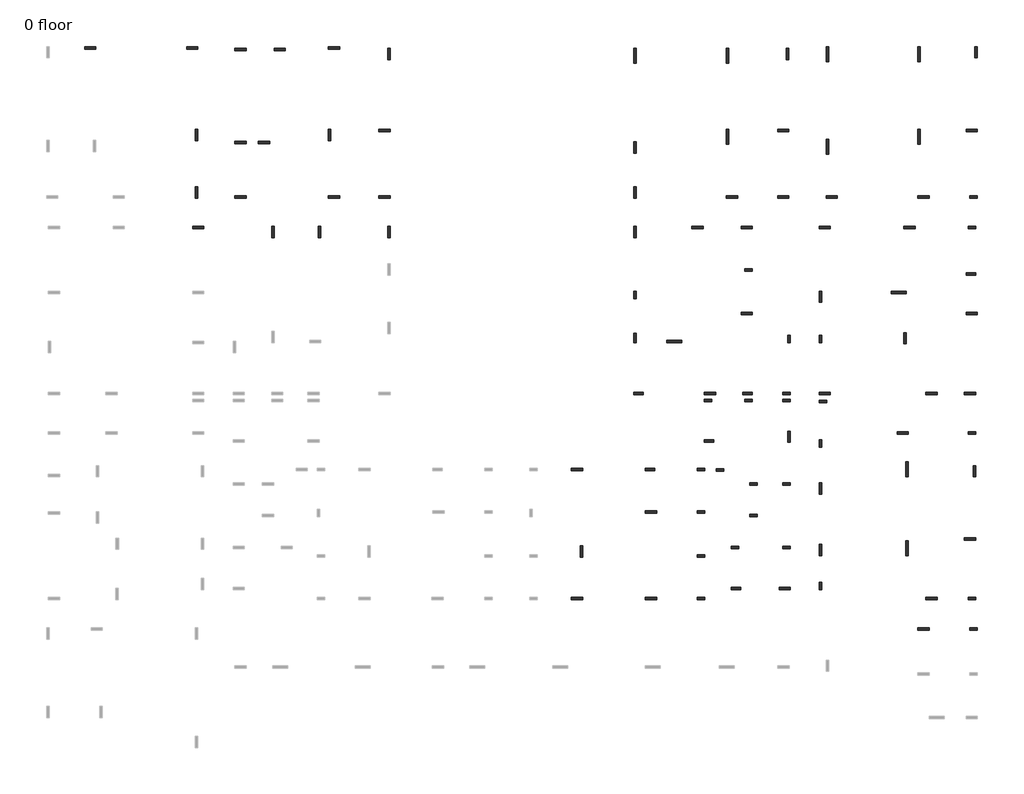
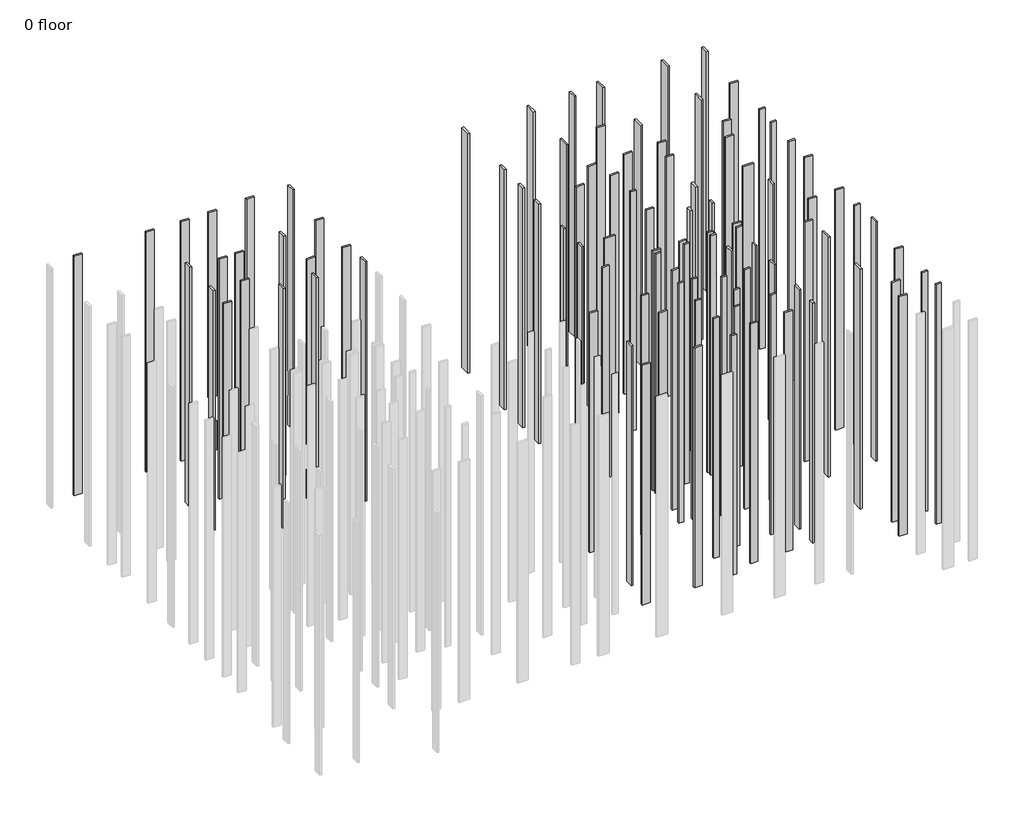
# One storey, part 2 of 2: 100 columns.
"""IFC4 building model written with IfcOpenShell, lengths in millimetres."""

from ifc_helpers import new_model, si_unit, frame, origin, origin_with_axes, place, context, project, spatial, polyline, outline, extrude, faceted_brep, transform, mapped, element, save
from components import column_6d4d5e46, column_25705251, column_7936e864, column_a28f250a

model = new_model("IFC4")

# Units and contexts
model_context = context("Model", 3, world=origin())
ifc_project = project(units=[si_unit("LENGTHUNIT", "METRE", prefix="MILLI")], contexts=[model_context])

# Site, building, storey
site = spatial("IfcSite", under=ifc_project)
building = spatial("IfcBuilding", under=site)
storey = spatial("IfcBuildingStorey", under=building, Name="0 floor", Elevation=0.0)

# Columns
placement = place(None, origin())
column_shape = column_6d4d5e46(model_context)
element("IfcColumn", 1, ObjectType="Rectangular Column : 2' x 8\"", at=placement, inside=storey, context=model_context, shape_type="MappedRepresentation", body=[
    mapped(column_shape, transform((32806.420549, 1766.0930615, 0.0), x_axis=(1.0, 0.0, 0.0), y_axis=(0.0, 1.0, 0.0), z_axis=(0.0, 0.0, 1.0))),
])
element("IfcColumn", 2, ObjectType="Rectangular Column : 2' x 8\"", at=placement, inside=storey, context=model_context, shape_type="MappedRepresentation", body=[
    mapped(column_shape, transform((10708.4180594, 14707.393062, 0.0), x_axis=(1.0, 0.0, 0.0), y_axis=(0.0, 1.0, 0.0), z_axis=(0.0, 0.0, 1.0))),
])
element("IfcColumn", 3, ObjectType="Rectangular Column : 2' x 8\"", at=placement, inside=storey, context=model_context, shape_type="MappedRepresentation", body=[
    mapped(column_shape, transform((10708.420549, 11265.693062, 0.0), x_axis=(-1.0, 0.0, 0.0), y_axis=(0.0, -1.0, 0.0), z_axis=(0.0, 0.0, 1.0))),
])
element("IfcColumn", 4, ObjectType="Rectangular Column : 2' x 8\"", at=placement, inside=storey, context=model_context, shape_type="MappedRepresentation", body=[
    mapped(column_shape, transform((10708.420549, 4255.2930586, 0.0), x_axis=(-1.0, 0.0, 0.0), y_axis=(0.0, -1.0, 0.0), z_axis=(0.0, 0.0, 1.0))),
])
element("IfcColumn", 5, ObjectType="Rectangular Column : 2' x 8\"", at=placement, inside=storey, context=model_context, shape_type="MappedRepresentation", body=[
    mapped(column_shape, transform((10708.420549, 7709.5953697, 0.0), x_axis=(-1.0, 0.0, 0.0), y_axis=(0.0, -1.0, 0.0), z_axis=(0.0, 0.0, 1.0))),
])
element("IfcColumn", 6, ObjectType="Rectangular Column : 2' x 8\"", at=placement, inside=storey, context=model_context, shape_type="MappedRepresentation", body=[
    mapped(column_shape, transform((13454.4520067, 8408.1930618, 0.0), x_axis=(1.0, 0.0, 0.0), y_axis=(0.0, 1.0, 0.0), z_axis=(0.0, 0.0, 1.0))),
])
element("IfcColumn", 7, ObjectType="Rectangular Column : 2' x 8\"", at=placement, inside=storey, context=model_context, shape_type="MappedRepresentation", body=[
    mapped(column_shape, transform((17645.4520067, 8408.1930618, 0.0), x_axis=(1.0, 0.0, 0.0), y_axis=(0.0, 1.0, 0.0), z_axis=(0.0, 0.0, 1.0))),
])
element("IfcColumn", 8, ObjectType="Rectangular Column : 2' x 8\"", at=placement, inside=storey, context=model_context, shape_type="MappedRepresentation", body=[
    mapped(column_shape, transform((14962.920549, 13538.9930617, 0.0), x_axis=(1.0, 0.0, 0.0), y_axis=(0.0, 1.0, 0.0), z_axis=(0.0, 0.0, 1.0))),
])
element("IfcColumn", 9, ObjectType="Rectangular Column : 2' x 8\"", at=placement, inside=storey, context=model_context, shape_type="MappedRepresentation", body=[
    mapped(column_shape, transform((14962.920549, 10986.2930571, 0.0), x_axis=(1.0, 0.0, 0.0), y_axis=(0.0, 1.0, 0.0), z_axis=(0.0, 0.0, 1.0))),
])
element("IfcColumn", 10, ObjectType="Rectangular Column : 2' x 8\"", at=placement, inside=storey, context=model_context, shape_type="MappedRepresentation", body=[
    mapped(column_shape, transform((17645.4520067, 13538.9930617, 0.0), x_axis=(1.0, 0.0, 0.0), y_axis=(0.0, 1.0, 0.0), z_axis=(0.0, 0.0, 1.0))),
])
element("IfcColumn", 11, ObjectType="Rectangular Column : 2' x 8\"", at=placement, inside=storey, context=model_context, shape_type="MappedRepresentation", body=[
    mapped(column_shape, transform((12235.2520067, 14681.993062, 0.0), x_axis=(1.0, 0.0, 0.0), y_axis=(0.0, 1.0, 0.0), z_axis=(0.0, 0.0, 1.0))),
])
element("IfcColumn", 12, ObjectType="Rectangular Column : 2' x 8\"", at=placement, inside=storey, context=model_context, shape_type="MappedRepresentation", body=[
    mapped(column_shape, transform((11282.7520067, 20308.093062, 0.0), x_axis=(1.0, 0.0, 0.0), y_axis=(0.0, 1.0, 0.0), z_axis=(0.0, 0.0, 1.0))),
])
element("IfcColumn", 13, ObjectType="Rectangular Column : 2' x 8\"", at=placement, inside=storey, context=model_context, shape_type="MappedRepresentation", body=[
    mapped(column_shape, transform((14556.520549, 20308.093062, 0.0), x_axis=(1.0, 0.0, 0.0), y_axis=(0.0, 1.0, 0.0), z_axis=(0.0, 0.0, 1.0))),
])
element("IfcColumn", 14, ObjectType="Rectangular Column : 2' x 8\"", at=placement, inside=storey, context=model_context, shape_type="MappedRepresentation", body=[
    mapped(column_shape, transform((17642.6205489, 20892.2930623, 0.0), x_axis=(1.0, 0.0, 0.0), y_axis=(0.0, 1.0, 0.0), z_axis=(0.0, 0.0, 1.0))),
])
element("IfcColumn", 15, ObjectType="Rectangular Column : 2' x 8\"", at=placement, inside=storey, context=model_context, shape_type="MappedRepresentation", body=[
    mapped(column_shape, transform((17642.618059, 20308.093062, 0.0), x_axis=(1.0, 0.0, 0.0), y_axis=(0.0, 1.0, 0.0), z_axis=(0.0, 0.0, 1.0))),
])
element("IfcColumn", 16, ObjectType="Rectangular Column : 2' x 8\"", at=placement, inside=storey, context=model_context, shape_type="MappedRepresentation", body=[
    mapped(column_shape, transform((5361.720549, 28867.8930624, 0.0), x_axis=(0.0, 1.0, 0.0), y_axis=(-1.0, 0.0, 0.0), z_axis=(0.0, 0.0, 1.0))),
])
element("IfcColumn", 17, ObjectType="Rectangular Column : 2' x 8\"", at=placement, inside=storey, context=model_context, shape_type="MappedRepresentation", body=[
    mapped(column_shape, transform((14556.520549, 30899.893062, 0.0), x_axis=(1.0, 0.0, 0.0), y_axis=(0.0, 1.0, 0.0), z_axis=(0.0, 0.0, 1.0))),
])
element("IfcColumn", 18, ObjectType="Rectangular Column : 2' x 8\"", at=placement, inside=storey, context=model_context, shape_type="MappedRepresentation", body=[
    mapped(column_shape, transform((17845.820549, 25311.8930465, 0.0), x_axis=(0.0, 1.0, 0.0), y_axis=(-1.0, 0.0, 0.0), z_axis=(0.0, 0.0, 1.0))),
])
element("IfcColumn", 19, ObjectType="Rectangular Column : 2' x 8\"", at=placement, inside=storey, context=model_context, shape_type="MappedRepresentation", body=[
    mapped(column_shape, transform((32654.0205491, 4255.2930626, 0.0), x_axis=(1.0, 0.0, 0.0), y_axis=(0.0, 1.0, 0.0), z_axis=(0.0, 0.0, 1.0))),
])
element("IfcColumn", 20, ObjectType="Rectangular Column : 2' x 8\"", at=placement, inside=storey, context=model_context, shape_type="MappedRepresentation", body=[
    mapped(column_shape, transform((32654.020549, 17679.1930626, 0.0), x_axis=(1.0, 0.0, 0.0), y_axis=(0.0, 1.0, 0.0), z_axis=(0.0, 0.0, 1.0))),
])
element("IfcColumn", 21, ObjectType="Rectangular Column : 2' x 8\"", at=placement, inside=storey, context=model_context, shape_type="MappedRepresentation", body=[
    mapped(column_shape, transform((32654.0205491, 34316.1930593, 0.0), x_axis=(1.0, 0.0, 0.0), y_axis=(0.0, 1.0, 0.0), z_axis=(0.0, 0.0, 1.0))),
])
element("IfcColumn", 22, ObjectType="Rectangular Column : 2' x 8\"", at=placement, inside=storey, context=model_context, shape_type="MappedRepresentation", body=[
    mapped(column_shape, transform((20586.1915809, 20244.5930606, 0.0), x_axis=(1.0, 0.0, 0.0), y_axis=(0.0, 1.0, 0.0), z_axis=(0.0, 0.0, 1.0))),
])
element("IfcColumn", 23, ObjectType="Rectangular Column : 2' x 8\"", at=placement, inside=storey, context=model_context, shape_type="MappedRepresentation", body=[
    mapped(column_shape, transform((20373.120549, 16802.893062, 0.0), x_axis=(0.0, 1.0, 0.0), y_axis=(-1.0, 0.0, 0.0), z_axis=(0.0, 0.0, 1.0))),
])
element("IfcColumn", 24, ObjectType="Rectangular Column : 2' x 8\"", at=placement, inside=storey, context=model_context, shape_type="MappedRepresentation", body=[
    mapped(column_shape, transform((20373.120549, 5283.9930634, 0.0), x_axis=(0.0, 1.0, 0.0), y_axis=(-1.0, 0.0, 0.0), z_axis=(0.0, 0.0, 1.0))),
])
element("IfcColumn", 25, ObjectType="Rectangular Column : 2' x 8\"", at=placement, inside=storey, context=model_context, shape_type="MappedRepresentation", body=[
    mapped(column_shape, transform((20373.120549, 25311.8930566, 0.0), x_axis=(0.0, 1.0, 0.0), y_axis=(-1.0, 0.0, 0.0), z_axis=(0.0, 0.0, 1.0))),
])
element("IfcColumn", 26, ObjectType="Rectangular Column : 2' x 8\"", at=placement, inside=storey, context=model_context, shape_type="MappedRepresentation", body=[
    mapped(column_shape, transform((32806.420549, 36805.393062, 0.0), x_axis=(1.0, 0.0, 0.0), y_axis=(0.0, 1.0, 0.0), z_axis=(0.0, 0.0, 1.0))),
])
column_2_shape = column_25705251(model_context)
element("IfcColumn", 27, ObjectType="Rectangular Column : 8\" x 2'6\"", at=placement, inside=storey, context=model_context, shape_type="MappedRepresentation", body=[
    mapped(column_2_shape, transform((6568.220549, 14706.9955039, 0.0), x_axis=(1.0, 0.0, 0.0), y_axis=(0.0, 1.0, 0.0), z_axis=(0.0, 0.0, 1.0))),
])
element("IfcColumn", 28, ObjectType="Rectangular Column : 8\" x 2'6\"", at=placement, inside=storey, context=model_context, shape_type="MappedRepresentation", body=[
    mapped(column_2_shape, transform((13530.6520067, 5080.7930619, 0.0), x_axis=(1.0, 0.0, 0.0), y_axis=(0.0, 1.0, 0.0), z_axis=(0.0, 0.0, 1.0))),
])
element("IfcColumn", 29, ObjectType="Rectangular Column : 8\" x 2'6\"", at=placement, inside=storey, context=model_context, shape_type="MappedRepresentation", body=[
    mapped(column_2_shape, transform((11358.9520067, 17006.093062, 0.0), x_axis=(1.0, 0.0, 0.0), y_axis=(0.0, 1.0, 0.0), z_axis=(0.0, 0.0, 1.0))),
])
element("IfcColumn", 30, ObjectType="Rectangular Column : 8\" x 2'6\"", at=placement, inside=storey, context=model_context, shape_type="MappedRepresentation", body=[
    mapped(column_2_shape, transform((14480.3205488, 20892.2930623, 0.0), x_axis=(1.0, 0.0, 0.0), y_axis=(0.0, 1.0, 0.0), z_axis=(0.0, 0.0, 1.0))),
])
element("IfcColumn", 31, ObjectType="Rectangular Column : 8\" x 2'6\"", at=placement, inside=storey, context=model_context, shape_type="MappedRepresentation", body=[
    mapped(column_2_shape, transform((5361.720549, 25388.093059, 0.0), x_axis=(0.0, 1.0, 0.0), y_axis=(-1.0, 0.0, 0.0), z_axis=(0.0, 0.0, 1.0))),
])
element("IfcColumn", 32, ObjectType="Rectangular Column : 8\" x 2'6\"", at=placement, inside=storey, context=model_context, shape_type="MappedRepresentation", body=[
    mapped(column_2_shape, transform((5641.120549, 20892.2930623, 0.0), x_axis=(-1.0, 0.0, 0.0), y_axis=(0.0, -1.0, 0.0), z_axis=(0.0, 0.0, 1.0))),
])
element("IfcColumn", 33, ObjectType="Rectangular Column : 8\" x 2'6\"", at=placement, inside=storey, context=model_context, shape_type="MappedRepresentation", body=[
    mapped(column_2_shape, transform((32577.8205488, 30569.6930587, 0.0), x_axis=(1.0, 0.0, 0.0), y_axis=(0.0, 1.0, 0.0), z_axis=(0.0, 0.0, 1.0))),
])
element("IfcColumn", 34, ObjectType="Rectangular Column : 8\" x 3'", at=placement, inside=storey, context=model_context, shape_type="SweptSolid", body=[
    extrude(outline(polyline([(-23004.2428642, 48850.8496871), (-23004.2428642, 48647.6496871), (-23918.6428642, 48647.6496871), (-23918.6428642, 48850.8496871), (-23004.2428642, 48850.8496871)])), origin_with_axes(), (0.0, 0.0, 1.0), 3505.2),
    extrude(outline(polyline([(-23004.2428642, 48850.8496871), (-23004.2428642, 48647.6496871), (-23918.6428642, 48647.6496871), (-23918.6428642, 48850.8496871), (-23004.2428642, 48850.8496871)])), frame((0.0, 0.0, 6553.2), z_axis=(0.0, 0.0, 1.0), x_axis=(1.0, 0.0, 0.0)), (0.0, 0.0, 1.0), 22555.2),
])
element("IfcColumn", 35, ObjectType="Rectangular Column : 8\" x 3'", at=placement, inside=storey, context=model_context, shape_type="Brep", body=[
    faceted_brep([(-26166.5159189, 48850.883515, 0.0), (-26166.5159189, 48647.683515, 0.0), (-27080.9159189, 48647.683515, 0.0), (-27080.9159189, 48850.883515, 0.0), (-26166.5159189, 48850.883515, 29108.4), (-26166.5159189, 48647.683515, 29108.4), (-26166.5159189, 48647.683515, 6553.2), (-26166.5159189, 48647.683515, 3505.2), (-26166.5159189, 48850.883515, 3505.2), (-26166.5159189, 48850.883515, 6553.2), (-27080.9159189, 48647.683515, 29108.4), (-27080.9159189, 48850.883515, 29108.4)], [[[0, 1, 2, 3]], [[4, 5, 6, 7, 1, 0, 8, 9]], [[5, 10, 2, 1, 7, 6]], [[10, 11, 3, 2]], [[11, 4, 9, 8, 0, 3]], [[4, 11, 10, 5]]]),
])
element("IfcColumn", 36, ObjectType="Rectangular Column : 8\" x 3'", at=placement, inside=storey, context=model_context, shape_type="Brep", body=[
    faceted_brep([(-18587.4473751, 49003.2834458, 0.0), (-18587.4473751, 48800.0834458, 0.0), (-19501.8473751, 48800.0834458, 0.0), (-19501.8473751, 49003.2834458, 0.0), (-18587.4473751, 49003.2834458, 29108.4), (-18587.4473751, 48800.0834458, 29108.4), (-19501.8473751, 48800.0834458, 29108.4), (-19501.8473751, 49003.2834458, 29108.4), (-19501.8473751, 49003.2834458, 6553.2), (-19501.8473751, 49003.2834458, 3505.2)], [[[0, 1, 2, 3]], [[4, 5, 1, 0]], [[5, 6, 2, 1]], [[6, 7, 8, 9, 3, 2]], [[7, 4, 0, 3, 9, 8]], [[4, 7, 6, 5]]]),
])
element("IfcColumn", 37, ObjectType="Rectangular Column : 8\" x 3'", at=placement, inside=storey, context=model_context, shape_type="Brep", body=[
    faceted_brep([(-14713.9473752, 48850.8834491, 0.0), (-14510.7473752, 48850.8834491, 0.0), (-14510.7473752, 47936.4834491, 0.0), (-14713.9473752, 47936.4834491, 0.0), (-14713.9473752, 48850.8834491, 29108.4), (-14510.7473752, 48850.8834491, 29108.4), (-14510.7473752, 48850.8834491, 6553.2), (-14713.9473752, 48850.8834491, 6553.2), (-14510.7473752, 48850.8834491, 3505.2), (-14510.7473752, 48749.2834491, 3505.2), (-14510.7473752, 48749.2834491, 6553.2), (-14510.7473752, 47936.4834491, 29108.4), (-14510.7473752, 47936.4834491, 6553.2), (-14510.7473752, 47936.4834491, 3505.2), (-14713.9473752, 47936.4834491, 29108.4), (-14713.9473752, 47936.4834491, 6553.2), (-14713.9473752, 47936.4834491, 3505.2), (-14713.9473752, 48749.2834491, 6553.2), (-14713.9473752, 48749.2834491, 3505.2), (-14713.9473752, 48850.8834491, 3505.2)], [[[0, 1, 2, 3]], [[4, 5, 6, 7]], [[2, 1, 8, 9, 10, 6, 5, 11, 12, 13]], [[3, 2, 13, 12, 11, 14, 15, 16]], [[0, 3, 16, 15, 14, 4, 7, 17, 18, 19]], [[5, 4, 14, 11]], [[18, 9, 8, 19]], [[10, 17, 7, 6]], [[9, 18, 17, 10]], [[1, 0, 19, 8]]]),
])
element("IfcColumn", 38, ObjectType="Rectangular Column : 8\" x 3'", at=placement, inside=storey, context=model_context, shape_type="Brep", body=[
    faceted_brep([(-19501.8473752, 42291.7930622, 0.0), (-19298.6473752, 42291.7930622, 0.0), (-19298.6473752, 41377.3930622, 0.0), (-19501.8473752, 41377.3930622, 0.0), (-19501.8473752, 42291.7930622, 29108.4), (-19298.6473752, 42291.7930622, 29108.4), (-19298.6473752, 41377.3930622, 29108.4), (-19501.8473752, 41377.3930622, 29108.4), (-19501.8473752, 41377.3930622, 6553.2), (-19501.8473752, 41377.3930622, 3505.2)], [[[0, 1, 2, 3]], [[4, 5, 1, 0]], [[5, 6, 2, 1]], [[6, 7, 8, 9, 3, 2]], [[7, 4, 0, 3, 9, 8]], [[4, 7, 6, 5]]]),
])
element("IfcColumn", 39, ObjectType="Rectangular Column : 8\" x 3'", at=placement, inside=storey, context=model_context, shape_type="Brep", body=[
    faceted_brep([(-27080.9159175, 41110.6930626, 0.0), (-27080.9159175, 41313.8930626, 0.0), (-26166.5159175, 41313.8930626, 0.0), (-26166.5159175, 41110.6930626, 0.0), (-27080.9159175, 41110.6930626, 29108.4), (-27080.9159175, 41313.8930626, 29108.4), (-27080.9159175, 41313.8930626, 6553.2), (-27080.9159175, 41313.8930626, 3505.2), (-27080.9159175, 41110.6930626, 3505.2), (-27080.9159175, 41110.6930626, 6553.2), (-26166.5159175, 41313.8930626, 29108.4), (-26166.5159175, 41110.6930626, 29108.4)], [[[0, 1, 2, 3]], [[4, 5, 6, 7, 1, 0, 8, 9]], [[5, 10, 2, 1, 7, 6]], [[10, 11, 3, 2]], [[11, 4, 9, 8, 0, 3]], [[4, 11, 10, 5]]]),
])
element("IfcColumn", 40, ObjectType="Rectangular Column : 8\" x 3'", at=placement, inside=storey, context=model_context, shape_type="Brep", body=[
    faceted_brep([(-25175.9159175, 41110.693059, 0.0), (-25175.9159175, 41313.893059, 0.0), (-24261.5159175, 41313.893059, 0.0), (-24261.5159175, 41110.693059, 0.0), (-25175.9159175, 41110.693059, 29108.4), (-25175.9159175, 41313.893059, 29108.4), (-25175.9159175, 41110.693059, 3505.2), (-25175.9159175, 41110.693059, 6553.2), (-24261.5159175, 41313.893059, 29108.4), (-24261.5159175, 41110.693059, 29108.4), (-24261.5159175, 41110.693059, 6553.2), (-24261.5159175, 41110.693059, 3505.2)], [[[0, 1, 2, 3]], [[4, 5, 1, 0, 6, 7]], [[5, 8, 2, 1]], [[8, 9, 10, 11, 3, 2]], [[9, 4, 7, 6, 0, 3, 11, 10]], [[4, 9, 8, 5]]]),
])
element("IfcColumn", 41, ObjectType="Rectangular Column : 8\" x 3'", at=placement, inside=storey, context=model_context, shape_type="Brep", body=[
    faceted_brep([(-15425.1473762, 42088.593059, 0.0), (-15425.1473762, 42291.793059, 0.0), (-14510.7473762, 42291.793059, 0.0), (-14510.7473762, 42088.593059, 0.0), (-15425.1473762, 42088.593059, 29108.4), (-15425.1473762, 42291.793059, 29108.4), (-15425.1473762, 42291.793059, 6553.2), (-15425.1473762, 42291.793059, 3505.2), (-14510.7473762, 42291.793059, 29108.4), (-14510.7473762, 42291.793059, 6553.2), (-14713.9473752, 42291.793059, 6553.2), (-14713.9473752, 42291.793059, 3505.2), (-14510.7473762, 42291.793059, 3505.2), (-14510.7473762, 42190.193059, 3505.2), (-14510.7473762, 42190.193059, 6553.2), (-14510.7473762, 42088.593059, 29108.4), (-14510.7473762, 42088.593059, 6553.2), (-14510.7473762, 42088.593059, 3505.2), (-14713.9473752, 42190.193059, 6553.2), (-14713.9473752, 42190.193059, 3505.2)], [[[0, 1, 2, 3]], [[1, 0, 4, 5, 6, 7]], [[2, 1, 7, 6, 5, 8, 9, 10, 11, 12]], [[3, 2, 12, 13, 14, 9, 8, 15, 16, 17]], [[0, 3, 17, 16, 15, 4]], [[5, 4, 15, 8]], [[18, 19, 11, 10]], [[19, 13, 12, 11]], [[14, 18, 10, 9]], [[19, 18, 14, 13]]]),
])
element("IfcColumn", 42, ObjectType="Rectangular Column : 8\" x 3'", at=placement, inside=storey, context=model_context, shape_type="Brep", body=[
    faceted_brep([(-15425.1473752, 36703.793059, 0.0), (-15425.1473752, 36906.993059, 0.0), (-14510.7473752, 36906.993059, 0.0), (-14510.7473752, 36703.793059, 0.0), (-15425.1473752, 36703.793059, 29108.4), (-15425.1473752, 36906.993059, 29108.4), (-15425.1473752, 36906.993059, 6553.2), (-15425.1473752, 36906.993059, 3505.2), (-15425.1473752, 36703.793059, 3505.2), (-15425.1473752, 36703.793059, 6553.2), (-14510.7473752, 36906.993059, 29108.4), (-14510.7473752, 36703.793059, 29108.4)], [[[0, 1, 2, 3]], [[4, 5, 6, 7, 1, 0, 8, 9]], [[5, 10, 2, 1, 7, 6]], [[10, 11, 3, 2]], [[11, 4, 9, 8, 0, 3]], [[4, 11, 10, 5]]]),
])
element("IfcColumn", 43, ObjectType="Rectangular Column : 8\" x 3'", at=placement, inside=storey, context=model_context, shape_type="Brep", body=[
    faceted_brep([(-19501.8473751, 36703.793059, 0.0), (-19501.8473751, 36906.993059, 0.0), (-18587.4473751, 36906.993059, 0.0), (-18587.4473751, 36703.793059, 0.0), (-19501.8473751, 36703.793059, 29108.4), (-19501.8473751, 36906.993059, 29108.4), (-19501.8473751, 36906.993059, 6553.2), (-19501.8473751, 36703.793059, 6553.2), (-19501.8473751, 36906.993059, 3505.2), (-19400.2473752, 36906.993059, 3505.2), (-19400.2473752, 36906.993059, 6553.2), (-18587.4473751, 36906.993059, 29108.4), (-18587.4473751, 36906.993059, 6553.2), (-18587.4473751, 36906.993059, 3505.2), (-18587.4473751, 36703.793059, 29108.4), (-18587.4473751, 36703.793059, 6553.2), (-18587.4473751, 36703.793059, 3505.2), (-19400.2473752, 36703.793059, 6553.2), (-19400.2473752, 36703.793059, 3505.2), (-19501.8473751, 36703.793059, 3505.2)], [[[0, 1, 2, 3]], [[4, 5, 6, 7]], [[2, 1, 8, 9, 10, 6, 5, 11, 12, 13]], [[3, 2, 13, 12, 11, 14, 15, 16]], [[0, 3, 16, 15, 14, 4, 7, 17, 18, 19]], [[5, 4, 14, 11]], [[18, 9, 8, 19]], [[10, 17, 7, 6]], [[9, 18, 17, 10]], [[1, 0, 19, 8]]]),
])
element("IfcColumn", 44, ObjectType="Rectangular Column : 8\" x 3'", at=placement, inside=storey, context=model_context, shape_type="Brep", body=[
    faceted_brep([(-27080.9159175, 36703.793059, 0.0), (-27080.9159175, 36906.993059, 0.0), (-26166.5159175, 36906.993059, 0.0), (-26166.5159175, 36703.793059, 0.0), (-27080.9159175, 36703.793059, 29108.4), (-27080.9159175, 36906.993059, 29108.4), (-27080.9159175, 36906.993059, 6553.2), (-27080.9159175, 36906.993059, 3505.2), (-26166.5159175, 36906.993059, 29108.4), (-26166.5159175, 36906.993059, 6553.2), (-26166.5159175, 36906.993059, 3505.2), (-26166.5159175, 36703.793059, 29108.4), (-26166.5159175, 36703.793059, 6553.2), (-26166.5159175, 36703.793059, 3505.2)], [[[0, 1, 2, 3]], [[4, 5, 6, 7, 1, 0]], [[5, 8, 9, 10, 2, 1, 7, 6]], [[8, 11, 12, 13, 3, 2, 10, 9]], [[11, 4, 0, 3, 13, 12]], [[4, 11, 8, 5]]]),
])
column_3_shape = column_7936e864(model_context)
element("IfcColumn", 45, ObjectType="Rectangular Column : 8\" x 3'", at=placement, inside=storey, context=model_context, shape_type="MappedRepresentation", body=[
    mapped(column_3_shape, transform((-30548.0159175, 48895.7926361, 0.0), x_axis=(1.0, 0.0, 0.0), y_axis=(0.0, 1.0, 0.0), z_axis=(0.0, 0.0, 1.0))),
])
element("IfcColumn", 46, ObjectType="Rectangular Column : 8\" x 3'", at=placement, inside=storey, context=model_context, shape_type="MappedRepresentation", body=[
    mapped(column_3_shape, transform((-38812.8844599, 48895.793059, 0.0), x_axis=(1.0, 0.0, 0.0), y_axis=(0.0, 1.0, 0.0), z_axis=(0.0, 0.0, 1.0))),
])
element("IfcColumn", 47, ObjectType="Rectangular Column : 8\" x 3'", at=placement, inside=storey, context=model_context, shape_type="MappedRepresentation", body=[
    mapped(column_3_shape, transform((-30192.4159175, 41834.5930622, 0.0), x_axis=(0.0, 1.0, 0.0), y_axis=(-1.0, 0.0, 0.0), z_axis=(0.0, 0.0, 1.0))),
])
element("IfcColumn", 48, ObjectType="Rectangular Column : 8\" x 3'", at=placement, inside=storey, context=model_context, shape_type="MappedRepresentation", body=[
    mapped(column_3_shape, transform((-30192.4159175, 37160.993059, 0.0), x_axis=(0.0, -1.0, 0.0), y_axis=(1.0, 0.0, 0.0), z_axis=(0.0, 0.0, 1.0))),
])
element("IfcColumn", 49, ObjectType="Rectangular Column : 8\" x 3'", at=placement, inside=storey, context=model_context, shape_type="MappedRepresentation", body=[
    mapped(column_3_shape, transform((-30058.579451, 34316.1930586, 0.0), x_axis=(1.0, 0.0, 0.0), y_axis=(0.0, 1.0, 0.0), z_axis=(0.0, 0.0, 1.0))),
])
element("IfcColumn", 50, ObjectType="Rectangular Column : 8\" x 3'", at=placement, inside=storey, context=model_context, shape_type="MappedRepresentation", body=[
    mapped(column_3_shape, transform((-24010.3473751, 33960.5930622, 0.0), x_axis=(0.0, -1.0, 0.0), y_axis=(1.0, 0.0, 0.0), z_axis=(0.0, 0.0, 1.0))),
])
element("IfcColumn", 51, ObjectType="Rectangular Column : 8\" x 3'", at=placement, inside=storey, context=model_context, shape_type="MappedRepresentation", body=[
    mapped(column_3_shape, transform((-20213.0473751, 33960.5930622, 0.0), x_axis=(0.0, -1.0, 0.0), y_axis=(1.0, 0.0, 0.0), z_axis=(0.0, 0.0, 1.0))),
])
element("IfcColumn", 52, ObjectType="Rectangular Column : 8\" x 3'", at=placement, inside=storey, context=model_context, shape_type="MappedRepresentation", body=[
    mapped(column_3_shape, transform((-14612.3473751, 33960.5930622, 0.0), x_axis=(0.0, -1.0, 0.0), y_axis=(1.0, 0.0, 0.0), z_axis=(0.0, 0.0, 1.0))),
])
element("IfcColumn", 53, ObjectType="Rectangular Column : 8\" x 3'", at=placement, inside=storey, context=model_context, shape_type="MappedRepresentation", body=[
    mapped(column_3_shape, transform((28729.720549, 1766.0930615, 0.0), x_axis=(1.0, 0.0, 0.0), y_axis=(0.0, 1.0, 0.0), z_axis=(0.0, 0.0, 1.0))),
])
element("IfcColumn", 54, ObjectType="Rectangular Column : 8\" x 3'", at=placement, inside=storey, context=model_context, shape_type="MappedRepresentation", body=[
    mapped(column_3_shape, transform((650.020549, 14707.393062, 0.0), x_axis=(-1.0, 0.0, 0.0), y_axis=(0.0, -1.0, 0.0), z_axis=(0.0, 0.0, 1.0))),
])
element("IfcColumn", 55, ObjectType="Rectangular Column : 8\" x 3'", at=placement, inside=storey, context=model_context, shape_type="MappedRepresentation", body=[
    mapped(column_3_shape, transform((1005.620549, 8065.2930636, 0.0), x_axis=(0.0, -1.0, 0.0), y_axis=(1.0, 0.0, 0.0), z_axis=(0.0, 0.0, 1.0))),
])
element("IfcColumn", 56, ObjectType="Rectangular Column : 8\" x 3'", at=placement, inside=storey, context=model_context, shape_type="MappedRepresentation", body=[
    mapped(column_3_shape, transform((650.0205489, 4255.293062, 0.0), x_axis=(1.0, 0.0, 0.0), y_axis=(0.0, 1.0, 0.0), z_axis=(0.0, 0.0, 1.0))),
])
element("IfcColumn", 57, ObjectType="Rectangular Column : 8\" x 3'", at=placement, inside=storey, context=model_context, shape_type="MappedRepresentation", body=[
    mapped(column_3_shape, transform((6644.4205495, 4255.2930614, 0.0), x_axis=(1.0, 0.0, 0.0), y_axis=(0.0, 1.0, 0.0), z_axis=(0.0, 0.0, 1.0))),
])
element("IfcColumn", 58, ObjectType="Rectangular Column : 8\" x 3'", at=placement, inside=storey, context=model_context, shape_type="MappedRepresentation", body=[
    mapped(column_3_shape, transform((6647.2520062, 11265.693062, 0.0), x_axis=(1.0, 0.0, 0.0), y_axis=(0.0, 1.0, 0.0), z_axis=(0.0, 0.0, 1.0))),
])
element("IfcColumn", 59, ObjectType="Rectangular Column : 8\" x 3'", at=placement, inside=storey, context=model_context, shape_type="MappedRepresentation", body=[
    mapped(column_3_shape, transform((17493.0520067, 5080.7930619, 0.0), x_axis=(1.0, 0.0, 0.0), y_axis=(0.0, 1.0, 0.0), z_axis=(0.0, 0.0, 1.0))),
])
element("IfcColumn", 60, ObjectType="Rectangular Column : 8\" x 3'", at=placement, inside=storey, context=model_context, shape_type="MappedRepresentation", body=[
    mapped(column_3_shape, transform((11432.3180598, 20892.2930623, 0.0), x_axis=(1.0, 0.0, 0.0), y_axis=(0.0, 1.0, 0.0), z_axis=(0.0, 0.0, 1.0))),
])
element("IfcColumn", 61, ObjectType="Rectangular Column : 8\" x 3'", at=placement, inside=storey, context=model_context, shape_type="MappedRepresentation", body=[
    mapped(column_3_shape, transform((17845.820549, 17361.6930611, 0.0), x_axis=(0.0, 1.0, 0.0), y_axis=(-1.0, 0.0, 0.0), z_axis=(0.0, 0.0, 1.0))),
])
element("IfcColumn", 62, ObjectType="Rectangular Column : 8\" x 3'", at=placement, inside=storey, context=model_context, shape_type="MappedRepresentation", body=[
    mapped(column_3_shape, transform((14404.9814343, 27342.8846086, 0.0), x_axis=(-1.0, 0.0, 0.0), y_axis=(0.0, -1.0, 0.0), z_axis=(0.0, 0.0, 1.0))),
])
element("IfcColumn", 63, ObjectType="Rectangular Column : 8\" x 3'", at=placement, inside=storey, context=model_context, shape_type="MappedRepresentation", body=[
    mapped(column_3_shape, transform((14404.1205491, 34316.1930612, 0.0), x_axis=(-1.0, 0.0, 0.0), y_axis=(0.0, -1.0, 0.0), z_axis=(0.0, 0.0, 1.0))),
])
element("IfcColumn", 64, ObjectType="Rectangular Column : 8\" x 3'", at=placement, inside=storey, context=model_context, shape_type="MappedRepresentation", body=[
    mapped(column_3_shape, transform((10403.620549, 34315.616008, 0.0), x_axis=(-1.0, 0.0, 0.0), y_axis=(0.0, -1.0, 0.0), z_axis=(0.0, 0.0, 1.0))),
])
element("IfcColumn", 65, ObjectType="Rectangular Column : 8\" x 3'", at=placement, inside=storey, context=model_context, shape_type="MappedRepresentation", body=[
    mapped(column_3_shape, transform((5361.720549, 33960.5930795, 0.0), x_axis=(0.0, -1.0, 0.0), y_axis=(1.0, 0.0, 0.0), z_axis=(0.0, 0.0, 1.0))),
])
element("IfcColumn", 66, ObjectType="Rectangular Column : 8\" x 3'", at=placement, inside=storey, context=model_context, shape_type="MappedRepresentation", body=[
    mapped(column_3_shape, transform((29377.420549, 4255.2930632, 0.0), x_axis=(1.0, 0.0, 0.0), y_axis=(0.0, 1.0, 0.0), z_axis=(0.0, 0.0, 1.0))),
])
element("IfcColumn", 67, ObjectType="Rectangular Column : 8\" x 3'", at=placement, inside=storey, context=model_context, shape_type="MappedRepresentation", body=[
    mapped(column_3_shape, transform((32501.6205491, 9093.9930626, 0.0), x_axis=(1.0, 0.0, 0.0), y_axis=(0.0, 1.0, 0.0), z_axis=(0.0, 0.0, 1.0))),
])
element("IfcColumn", 68, ObjectType="Rectangular Column : 8\" x 3'", at=placement, inside=storey, context=model_context, shape_type="MappedRepresentation", body=[
    mapped(column_3_shape, transform((32857.2205491, 14580.3930621, 0.0), x_axis=(0.0, 1.0, 0.0), y_axis=(-1.0, 0.0, 0.0), z_axis=(0.0, 0.0, 1.0))),
])
element("IfcColumn", 69, ObjectType="Rectangular Column : 8\" x 3'", at=placement, inside=storey, context=model_context, shape_type="MappedRepresentation", body=[
    mapped(column_3_shape, transform((27053.320549, 17679.1930621, 0.0), x_axis=(-1.0, 0.0, 0.0), y_axis=(0.0, -1.0, 0.0), z_axis=(0.0, 0.0, 1.0))),
])
element("IfcColumn", 70, ObjectType="Rectangular Column : 8\" x 3'", at=placement, inside=storey, context=model_context, shape_type="MappedRepresentation", body=[
    mapped(column_3_shape, transform((27599.4205457, 34316.1930593, 0.0), x_axis=(1.0, 0.0, 0.0), y_axis=(0.0, 1.0, 0.0), z_axis=(0.0, 0.0, 1.0))),
])
element("IfcColumn", 71, ObjectType="Rectangular Column : 8\" x 3'", at=placement, inside=storey, context=model_context, shape_type="MappedRepresentation", body=[
    mapped(column_3_shape, transform((32654.020549, 27342.8846085, 0.0), x_axis=(1.0, 0.0, 0.0), y_axis=(0.0, 1.0, 0.0), z_axis=(0.0, 0.0, 1.0))),
])
element("IfcColumn", 72, ObjectType="Rectangular Column : 8\" x 3'", at=placement, inside=storey, context=model_context, shape_type="MappedRepresentation", body=[
    mapped(column_3_shape, transform((27243.8205478, 25362.693062, 0.0), x_axis=(0.0, 1.0, 0.0), y_axis=(-1.0, 0.0, 0.0), z_axis=(0.0, 0.0, 1.0))),
])
element("IfcColumn", 73, ObjectType="Rectangular Column : 8\" x 3'", at=placement, inside=storey, context=model_context, shape_type="MappedRepresentation", body=[
    mapped(column_3_shape, transform((29377.420549, 20892.293062, 0.0), x_axis=(-1.0, 0.0, 0.0), y_axis=(0.0, -1.0, 0.0), z_axis=(0.0, 0.0, 1.0))),
])
element("IfcColumn", 74, ObjectType="Rectangular Column : 8\" x 3'", at=placement, inside=storey, context=model_context, shape_type="MappedRepresentation", body=[
    mapped(column_3_shape, transform((32501.6205491, 20892.293062, 0.0), x_axis=(-1.0, 0.0, 0.0), y_axis=(0.0, -1.0, 0.0), z_axis=(0.0, 0.0, 1.0))),
])
element("IfcColumn", 75, ObjectType="Rectangular Column : 8\" x 3'", at=placement, inside=storey, context=model_context, shape_type="MappedRepresentation", body=[
    mapped(column_3_shape, transform((20728.7180591, 20892.2930623, 0.0), x_axis=(-1.0, 0.0, 0.0), y_axis=(0.0, -1.0, 0.0), z_axis=(0.0, 0.0, 1.0))),
])
element("IfcColumn", 76, ObjectType="Rectangular Column : 8\" x 3'", at=placement, inside=storey, context=model_context, shape_type="MappedRepresentation", body=[
    mapped(column_3_shape, transform((20373.120549, 13183.3930617, 0.0), x_axis=(0.0, 1.0, 0.0), y_axis=(-1.0, 0.0, 0.0), z_axis=(0.0, 0.0, 1.0))),
])
element("IfcColumn", 77, ObjectType="Rectangular Column : 8\" x 3'", at=placement, inside=storey, context=model_context, shape_type="MappedRepresentation", body=[
    mapped(column_3_shape, transform((20373.1180591, 8179.5930621, 0.0), x_axis=(0.0, 1.0, 0.0), y_axis=(-1.0, 0.0, 0.0), z_axis=(0.0, 0.0, 1.0))),
])
element("IfcColumn", 78, ObjectType="Rectangular Column : 8\" x 3'", at=placement, inside=storey, context=model_context, shape_type="MappedRepresentation", body=[
    mapped(column_3_shape, transform((20373.120549, 28715.493059, 0.0), x_axis=(0.0, 1.0, 0.0), y_axis=(-1.0, 0.0, 0.0), z_axis=(0.0, 0.0, 1.0))),
])
element("IfcColumn", 79, ObjectType="Rectangular Column : 8\" x 3'", at=placement, inside=storey, context=model_context, shape_type="MappedRepresentation", body=[
    mapped(column_3_shape, transform((20728.720549, 34316.1930644, 0.0), x_axis=(-1.0, 0.0, 0.0), y_axis=(0.0, -1.0, 0.0), z_axis=(0.0, 0.0, 1.0))),
])
element("IfcColumn", 80, ObjectType="Rectangular Column : 8\" x 3'", at=placement, inside=storey, context=model_context, shape_type="MappedRepresentation", body=[
    mapped(column_3_shape, transform((21300.2205485, 36805.393062, 0.0), x_axis=(1.0, 0.0, 0.0), y_axis=(0.0, 1.0, 0.0), z_axis=(0.0, 0.0, 1.0))),
])
element("IfcColumn", 81, ObjectType="Rectangular Column : 8\" x 3'", at=placement, inside=storey, context=model_context, shape_type="MappedRepresentation", body=[
    mapped(column_3_shape, transform((17375.3328031, 36805.393062, 0.0), x_axis=(1.0, 0.0, 0.0), y_axis=(0.0, 1.0, 0.0), z_axis=(0.0, 0.0, 1.0))),
])
element("IfcColumn", 82, ObjectType="Rectangular Column : 8\" x 3'", at=placement, inside=storey, context=model_context, shape_type="MappedRepresentation", body=[
    mapped(column_3_shape, transform((13222.4328033, 36805.393062, 0.0), x_axis=(1.0, 0.0, 0.0), y_axis=(0.0, 1.0, 0.0), z_axis=(0.0, 0.0, 1.0))),
])
element("IfcColumn", 83, ObjectType="Rectangular Column : 8\" x 3'", at=placement, inside=storey, context=model_context, shape_type="MappedRepresentation", body=[
    mapped(column_3_shape, transform((5361.720549, 37160.993062, 0.0), x_axis=(0.0, 1.0, 0.0), y_axis=(-1.0, 0.0, 0.0), z_axis=(0.0, 0.0, 1.0))),
])
element("IfcColumn", 84, ObjectType="Rectangular Column : 8\" x 3'", at=placement, inside=storey, context=model_context, shape_type="MappedRepresentation", body=[
    mapped(column_3_shape, transform((5361.720549, 40818.593062, 0.0), x_axis=(0.0, 1.0, 0.0), y_axis=(-1.0, 0.0, 0.0), z_axis=(0.0, 0.0, 1.0))),
])
element("IfcColumn", 85, ObjectType="Rectangular Column : 8\" x 3'", at=placement, inside=storey, context=model_context, shape_type="MappedRepresentation", body=[
    mapped(column_3_shape, transform((17375.3328033, 42190.193059, 0.0), x_axis=(-1.0, 0.0, 0.0), y_axis=(0.0, -1.0, 0.0), z_axis=(0.0, 0.0, 1.0))),
])
element("IfcColumn", 86, ObjectType="Rectangular Column : 8\" x 3'", at=placement, inside=storey, context=model_context, shape_type="MappedRepresentation", body=[
    mapped(column_3_shape, transform((17730.9328033, 48393.6834493, 0.0), x_axis=(0.0, 1.0, 0.0), y_axis=(-1.0, 0.0, 0.0), z_axis=(0.0, 0.0, 1.0))),
])
element("IfcColumn", 87, ObjectType="Rectangular Column : 8\" x 3'", at=placement, inside=storey, context=model_context, shape_type="MappedRepresentation", body=[
    mapped(column_3_shape, transform((32654.020549, 42190.193059, 0.0), x_axis=(1.0, 0.0, 0.0), y_axis=(0.0, 1.0, 0.0), z_axis=(0.0, 0.0, 1.0))),
])
element("IfcColumn", 88, ObjectType="Rectangular Column : 8\" x 3'", at=placement, inside=storey, context=model_context, shape_type="MappedRepresentation", body=[
    mapped(column_3_shape, transform((28729.720549, 36805.393062, 0.0), x_axis=(1.0, 0.0, 0.0), y_axis=(0.0, 1.0, 0.0), z_axis=(0.0, 0.0, 1.0))),
])
element("IfcColumn", 89, ObjectType="Rectangular Column : 8\" x 3'", at=placement, inside=storey, context=model_context, shape_type="MappedRepresentation", body=[
    mapped(column_3_shape, transform((33009.6205485, 48540.193062, 0.0), x_axis=(0.0, 1.0, 0.0), y_axis=(-1.0, 0.0, 0.0), z_axis=(0.0, 0.0, 1.0))),
])
column_4_shape = column_a28f250a(model_context)
element("IfcColumn", 90, ObjectType="Rectangular Column : 8\" x 4'", at=placement, inside=storey, context=model_context, shape_type="MappedRepresentation", body=[
    mapped(column_4_shape, transform((8536.720549, 25108.693059, 0.0), x_axis=(1.0, 0.0, 0.0), y_axis=(0.0, 1.0, 0.0), z_axis=(0.0, 0.0, 1.0))),
])
element("IfcColumn", 91, ObjectType="Rectangular Column : 8\" x 4'", at=placement, inside=storey, context=model_context, shape_type="MappedRepresentation", body=[
    mapped(column_4_shape, transform((27408.920549, 8331.9930621, 0.0), x_axis=(0.0, 1.0, 0.0), y_axis=(-1.0, 0.0, 0.0), z_axis=(0.0, 0.0, 1.0))),
])
element("IfcColumn", 92, ObjectType="Rectangular Column : 8\" x 4'", at=placement, inside=storey, context=model_context, shape_type="MappedRepresentation", body=[
    mapped(column_4_shape, transform((27408.920549, 14732.7930624, 0.0), x_axis=(0.0, 1.0, 0.0), y_axis=(-1.0, 0.0, 0.0), z_axis=(0.0, 0.0, 1.0))),
])
element("IfcColumn", 93, ObjectType="Rectangular Column : 8\" x 4'", at=placement, inside=storey, context=model_context, shape_type="MappedRepresentation", body=[
    mapped(column_4_shape, transform((26735.820549, 29071.093059, 0.0), x_axis=(1.0, 0.0, 0.0), y_axis=(0.0, 1.0, 0.0), z_axis=(0.0, 0.0, 1.0))),
])
element("IfcColumn", 94, ObjectType="Rectangular Column : 8\" x 4'", at=placement, inside=storey, context=model_context, shape_type="MappedRepresentation", body=[
    mapped(column_4_shape, transform((12866.8328033, 41682.193059, 0.0), x_axis=(0.0, 1.0, 0.0), y_axis=(-1.0, 0.0, 0.0), z_axis=(0.0, 0.0, 1.0))),
])
element("IfcColumn", 95, ObjectType="Rectangular Column : 8\" x 4'", at=placement, inside=storey, context=model_context, shape_type="MappedRepresentation", body=[
    mapped(column_4_shape, transform((5363.9642609, 48241.2834488, 0.0), x_axis=(0.0, 1.0, 0.0), y_axis=(-1.0, 0.0, 0.0), z_axis=(0.0, 0.0, 1.0))),
])
element("IfcColumn", 96, ObjectType="Rectangular Column : 8\" x 4'", at=placement, inside=storey, context=model_context, shape_type="MappedRepresentation", body=[
    mapped(column_4_shape, transform((12866.8328038, 48241.2834493, 0.0), x_axis=(0.0, 1.0, 0.0), y_axis=(-1.0, 0.0, 0.0), z_axis=(0.0, 0.0, 1.0))),
])
element("IfcColumn", 97, ObjectType="Rectangular Column : 8\" x 4'", at=placement, inside=storey, context=model_context, shape_type="MappedRepresentation", body=[
    mapped(column_4_shape, transform((20944.620549, 40869.3930594, 0.0), x_axis=(0.0, 1.0, 0.0), y_axis=(-1.0, 0.0, 0.0), z_axis=(0.0, 0.0, 1.0))),
])
element("IfcColumn", 98, ObjectType="Rectangular Column : 8\" x 4'", at=placement, inside=storey, context=model_context, shape_type="MappedRepresentation", body=[
    mapped(column_4_shape, transform((28374.120549, 41682.19318, 0.0), x_axis=(0.0, 1.0, 0.0), y_axis=(-1.0, 0.0, 0.0), z_axis=(0.0, 0.0, 1.0))),
])
element("IfcColumn", 99, ObjectType="Rectangular Column : 8\" x 4'", at=placement, inside=storey, context=model_context, shape_type="MappedRepresentation", body=[
    mapped(column_4_shape, transform((20944.620549, 48387.793062, 0.0), x_axis=(0.0, 1.0, 0.0), y_axis=(-1.0, 0.0, 0.0), z_axis=(0.0, 0.0, 1.0))),
])
element("IfcColumn", 100, ObjectType="Rectangular Column : 8\" x 4'", at=placement, inside=storey, context=model_context, shape_type="MappedRepresentation", body=[
    mapped(column_4_shape, transform((28374.1205485, 48387.793062, 0.0), x_axis=(0.0, 1.0, 0.0), y_axis=(-1.0, 0.0, 0.0), z_axis=(0.0, 0.0, 1.0))),
])

save(model, "model.ifc")

# Revit data of these elements
# Type "Rectangular Column : 2' x 8\""
#   Assembly Code = "B1010200"
#   Depth = 0' - 8"
#   Offset Base = 0' - 0"
#   Offset Top = 0' - 0"
#   Width = 2' - 0"
#   Material = none
# Type "Rectangular Column : 8\" x 2'6\""
#   Assembly Code = "B1010200"
#   Depth = 0' - 8"
#   Offset Base = 0' - 0"
#   Offset Top = 0' - 0"
#   Width = 2' - 6"
#   Material = none
# Type "Rectangular Column : 8\" x 3'"
#   Assembly Code = "B1010200"
#   Depth = 0' - 8"
#   Offset Base = 0' - 0"
#   Offset Top = 0' - 0"
#   Width = 3' - 0"
#   Material = none
# Type "Rectangular Column : 8\" x 4'"
#   Assembly Code = "B1010200"
#   Depth = 0' - 8"
#   Offset Base = 0' - 0"
#   Offset Top = 0' - 0"
#   Width = 4' - 0"
#   Material = none
# Elements 1, 2, 3, 4, 5, 6, 7, 8, 9, 10, 11, 12, 13, 14, 15, 16, 17, 18, 19, 20, 21, 22, 23, 24, 25, 26 (IfcColumn, "Rectangular Column : 2' x 8\"")
#   Phase Created = New Construction
# Elements 27, 28, 29, 30, 31, 32, 33 (IfcColumn, "Rectangular Column : 8\" x 2'6\"")
#   Phase Created = New Construction
# Elements 34, 35, 36, 37, 38, 39, 40, 41, 42, 43, 44 (IfcColumn, "Rectangular Column : 8\" x 3'")
#   Phase Created = New Construction
#   Materials on its faces: "00-8\" wall"
# Elements 45, 46, 47, 48, 49, 50, 51, 52, 53, 54, 55, 56, 57, 58, 59, 60, 61, 62, 63, 64, 65, 66, 67, 68, 69, 70, 71, 72, 73, 74, 75, 76, 77, 78, 79, 80, 81, 82, 83, 84, 85, 86, 87, 88, 89 (IfcColumn, "Rectangular Column : 8\" x 3'")
#   Phase Created = New Construction
# Elements 90, 91, 92, 93, 94, 95, 96, 97, 98, 99, 100 (IfcColumn, "Rectangular Column : 8\" x 4'")
#   Phase Created = New Construction
# Materials
#   "00-8\" wall": class "Generic", colour RGB 120 120 120, transparency 0, Cost = 0
